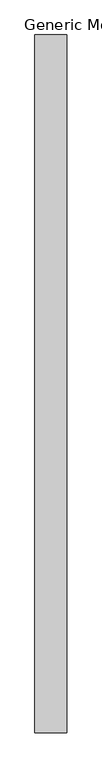
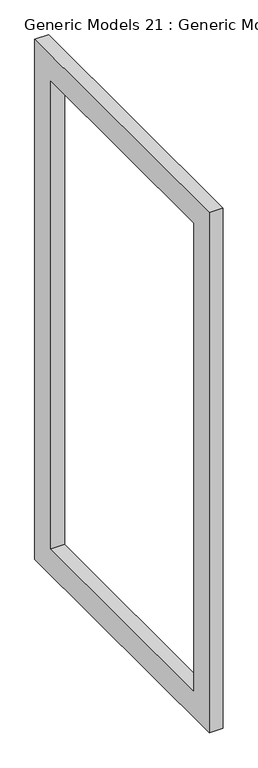
"""IFC4 building model written with IfcOpenShell, lengths in millimetres: proxy geometry, Generic Models 21 : Generic Models 23."""

from ifc_helpers import new_model, si_unit, frame, origin, place, context, project, spatial, polyline, outline, extrude, source, transform, mapped, element, save


def generic_models_21_generic_models_23_029173b4(model_context):
    return source(origin(), model_context, "Body", "SweptSolid", [
        extrude(outline(polyline([(6050.1857468, 9245.6), (7167.7857468, 9245.6), (7167.7857468, 7213.6), (6050.1857468, 7213.6), (6050.1857468, 9245.6)]), holes=[polyline([(6151.7857468, 9144.0), (6151.7857468, 7315.2), (7066.1857468, 7315.2), (7066.1857468, 9144.0), (6151.7857468, 9144.0)])]), frame((-10043.3781265, 0.0, 0.0), z_axis=(1.0, 0.0, 0.0), x_axis=(0.0, 1.0, 0.0)), (0.0, 0.0, 1.0), 50.8),
    ])


if __name__ == "__main__":
    model = new_model("IFC4")
    model_context = context("Model", 3, world=origin())
    ifc_project = project(units=[si_unit("LENGTHUNIT", "METRE", prefix="MILLI")], contexts=[model_context])
    site = spatial("IfcSite", under=ifc_project)
    building = spatial("IfcBuilding", under=site)
    placement = place(None, origin())
    generic_models_21_generic_models_23_shape = generic_models_21_generic_models_23_029173b4(model_context)
    element("IfcBuildingElementProxy", 1, Name="Generic Models 21 : Generic Models 23", ObjectType="Generic Models 21 : Generic Models 23", at=placement, inside=building, context=model_context, shape_type="MappedRepresentation", body=[
        mapped(generic_models_21_generic_models_23_shape, transform((0.0, 0.0, 0.0), x_axis=(1.0, 0.0, 0.0), y_axis=(0.0, 1.0, 0.0), z_axis=(0.0, 0.0, 1.0))),
    ])
    save(model, "model.ifc")
